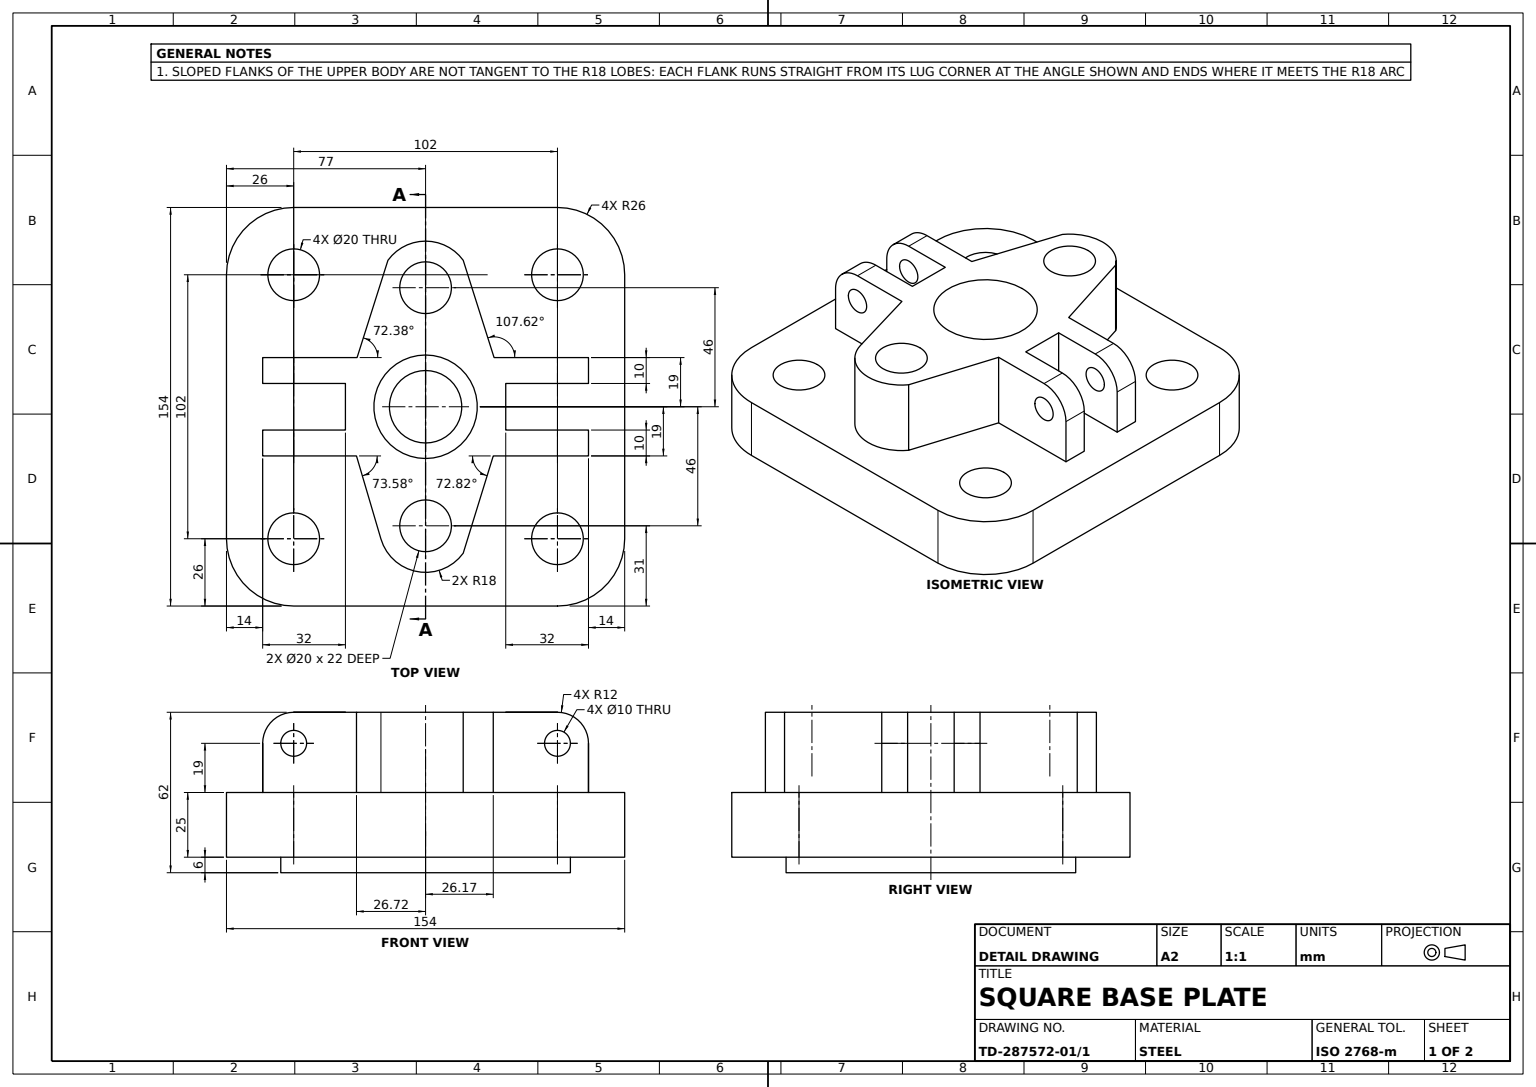
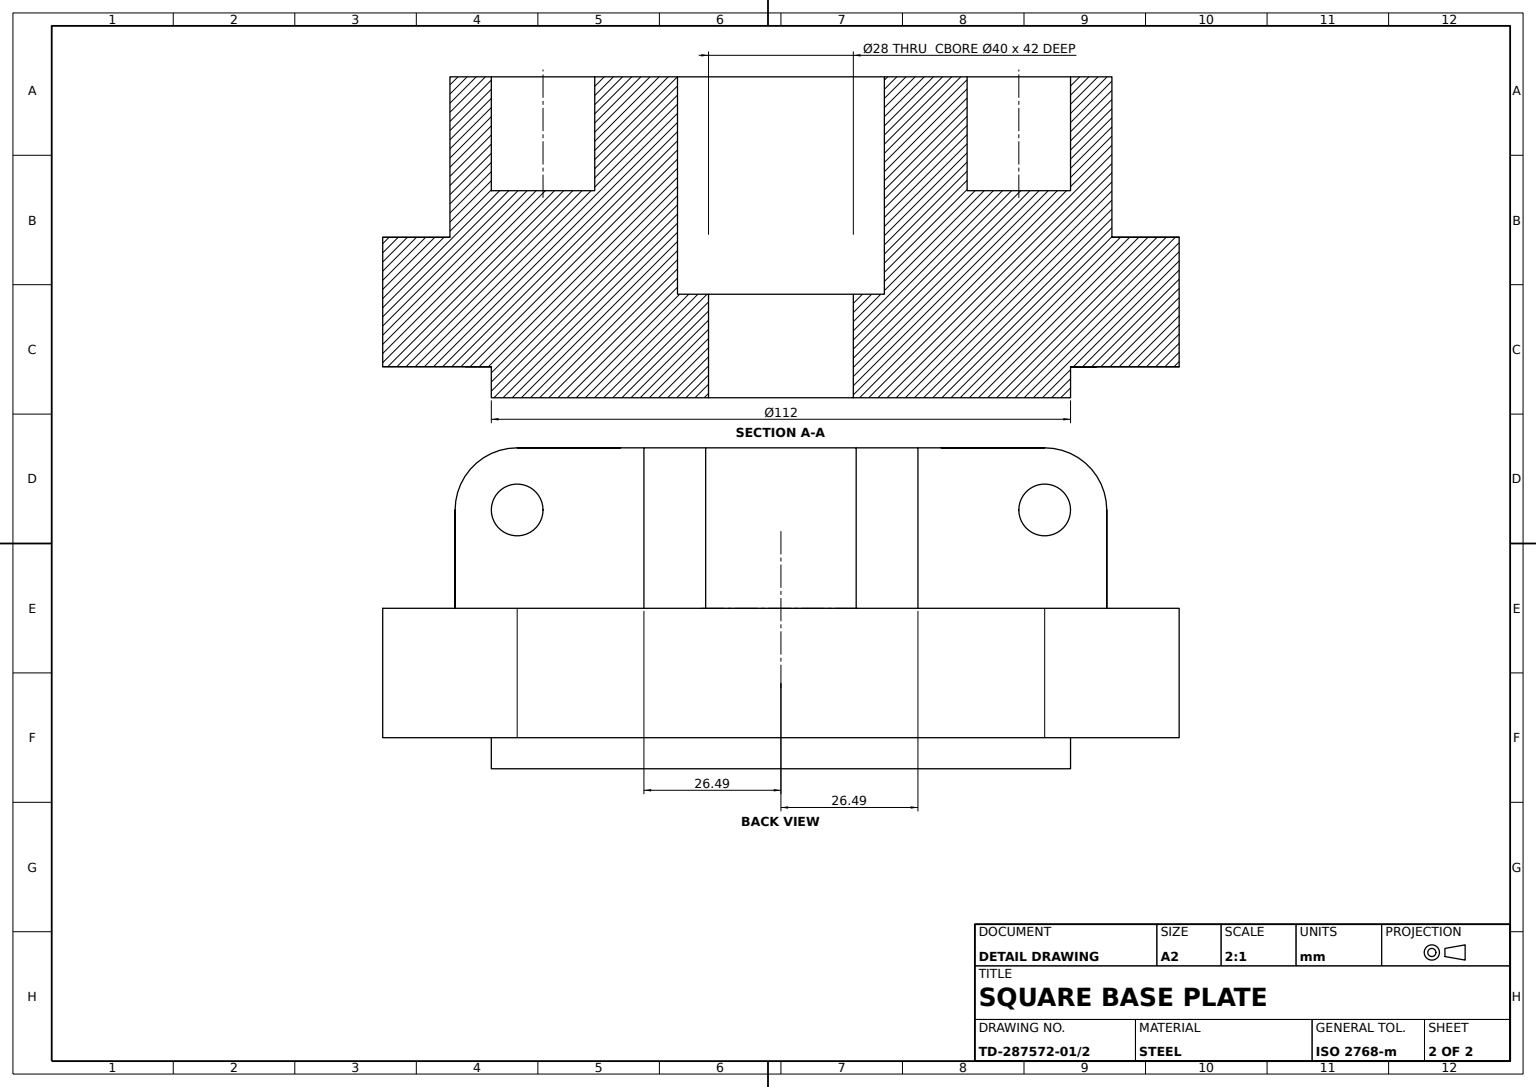
from build123d import *

# Parameters (mm, degrees)
BASE_PLATE_DEPTH              = 25
PLATE_MOUNTING_HOLES_SKETCH_R = 10
PLATE_MOUNTING_HOLES_DEPTH    = 112
CENTRAL_BOSS_DEPTH            = 31
LUG_START                     = -31
LUG_PAIR_A_DEPTH              = 31
LUG_PAIR_B_DEPTH              = 31
LUG_PIN_HOLES_SKETCH_R        = 5
LUG_PIN_HOLES_DEPTH           = 118
LUG_A_FILLET_1_R              = 12
LUG_A_FILLET_2_R              = 12
LUG_B_FILLET_1_R              = 12
LUG_B_FILLET_2_R              = 12
CENTRAL_BORE_SKETCH_R         = 14
CENTRAL_BORE_DEPTH            = 118
BORE_COUNTERBORE_SKETCH_R     = 20
BORE_COUNTERBORE_DEPTH        = 42
BOTTOM_SPIGOT_SKETCH_R        = 56
BOTTOM_SPIGOT_DEPTH           = 6
SPIGOT_BORE_SKETCH_R          = 14
SPIGOT_BORE_DEPTH             = 120
FLANGE_HOLE_1_SKETCH_R        = 10
FLANGE_HOLE_1_DEPTH           = 22
FLANGE_HOLE_2_SKETCH_R        = 10
FLANGE_HOLE_2_DEPTH           = 22


with BuildPart() as part:
    # Base Plate Sketch → Base Plate (new body)
    with BuildSketch(Plane(origin=(0, 0, 0), x_dir=(1, 0, 0), z_dir=(0, 1, 0))):
        with BuildLine():
            Line((77, 0), (77, 51))
            ThreePointArc((77, 51), (69.384776311, 69.384776311), (51, 77))
            Line((51, 77), (-51, 77))
            ThreePointArc((-51, 77), (-69.384776311, 69.384776311), (-77, 51))
            Line((-77, 51), (-77, -51))
            ThreePointArc((-77, -51), (-69.384776311, -69.384776311), (-51, -77))
            Line((-51, -77), (51, -77))
            ThreePointArc((51, -77), (69.384776311, -69.384776311), (77, -51))
            Line((77, -51), (77, 0))
        make_face()
    extrude(amount=BASE_PLATE_DEPTH)

    # Plate Mounting Holes Sketch → Plate Mounting Holes (cut)
    with BuildSketch(Plane(origin=(0, 25, 0), x_dir=(1, 0, 0), z_dir=(0, 1, 0))):
        with Locations(Location((-51, 51, 0), (0, 0, 270))):
            Circle(PLATE_MOUNTING_HOLES_SKETCH_R)
        with Locations(Location((51, 51, 0), (0, 0, 270))):
            Circle(PLATE_MOUNTING_HOLES_SKETCH_R)
        with Locations(Location((51, -51, 0), (0, 0, 270))):
            Circle(PLATE_MOUNTING_HOLES_SKETCH_R)
        with Locations(Location((-51, -51, 0), (0, 0, 270))):
            Circle(PLATE_MOUNTING_HOLES_SKETCH_R)
    extrude(amount=-PLATE_MOUNTING_HOLES_DEPTH, mode=Mode.SUBTRACT)

    # Central Boss Sketch → Central Boss (add)
    with BuildSketch(Plane(origin=(0, 25, 0), x_dir=(1, 0, 0), z_dir=(0, 1, 0))):
        with BuildLine():
            Line((14.551173168, 56.595440502), (29.545654505, 9.383725265))
            ThreePointArc((29.545654505, 9.383725265), (30.89470992, 2.552821763), (30.685167625, -4.406868258))
            Line((30.685167625, -4.406868258), (14.551173168, -56.595440502))
            ThreePointArc((14.551173168, -56.595440502), (-3.070625216, -63.736156878), (-17.266235066, -51.086956522))
            Line((-17.266235066, -51.086956522), (-29.736293724, -8.760869565))
            ThreePointArc((-29.736293724, -8.760869565), (-30.998289096, 0.325688707), (-29.545654505, 9.383725265))
            Line((-29.545654505, 9.383725265), (-14.551173168, 56.595440502))
            ThreePointArc((-14.551173168, 56.595440502), (0, 64), (14.551173168, 56.595440502))
        make_face()
    extrude(amount=CENTRAL_BOSS_DEPTH)

    # Lug Pair A Sketch → Lug Pair A (add)
    with BuildSketch(Plane(origin=(0, 56, 0), x_dir=(1, 0, 0), z_dir=(0, 1, 0)).offset(LUG_START)):
        with BuildLine():
            Line((31, 0), (31, 9))
            Line((31, 9), (63, 9))
            Line((63, 9), (63, 19))
            Line((63, 19), (31, 19))
            Line((31, 19), (26.491517384, 19))
            Line((26.491517384, 19), (29.545654505, 9.383725265))
            ThreePointArc((29.545654505, 9.383725265), (30.634256068, 4.747879018), (31, 0))
        make_face()
        with BuildLine():
            Line((31, -9), (31, 0))
            ThreePointArc((31, 0), (30.921191733, -2.209049981), (30.685167625, -4.406868258))
            ThreePointArc((30.685167625, -4.406868258), (29.6170045, -9.156038686), (27.818568264, -13.679446617))
            Line((27.818568264, -13.679446617), (26.173729651, -19))
            Line((26.173729651, -19), (31, -19))
            Line((31, -19), (63, -19))
            Line((63, -19), (63, -9))
            Line((63, -9), (31, -9))
        make_face()
        with BuildLine():
            ThreePointArc((24.494897428, 19), (27.444735347, 14.414801481), (29.545654505, 9.383725265))
            Line((29.545654505, 9.383725265), (26.491517384, 19))
            Line((26.491517384, 19), (24.494897428, 19))
        make_face()
        with BuildLine():
            Line((26.173729651, -19), (27.818568264, -13.679446617))
            ThreePointArc((27.818568264, -13.679446617), (26.29166684, -16.424014575), (24.494897428, -19))
            Line((24.494897428, -19), (26.173729651, -19))
        make_face()
        with BuildLine():
            ThreePointArc((27.818568264, -13.679446617), (29.6170045, -9.156038686), (30.685167625, -4.406868258))
            Line((30.685167625, -4.406868258), (27.818568264, -13.679446617))
        make_face()
    extrude(amount=LUG_PAIR_A_DEPTH)

    # Lug Pair B Sketch → Lug Pair B (add)
    with BuildSketch(Plane(origin=(0, 56, 0), x_dir=(1, 0, 0), z_dir=(0, 1, 0)).offset(LUG_START)):
        with BuildLine():
            ThreePointArc((-29.736293724, -8.760869565), (-30.682446981, -4.425770811), (-31, 0))
            Line((-31, 0), (-31, -9))
            Line((-31, -9), (-63, -9))
            Line((-63, -9), (-63, -19))
            Line((-63, -19), (-26.719653956, -19))
            Line((-26.719653956, -19), (-29.736293724, -8.760869565))
        make_face()
        with BuildLine():
            Line((-31, 9), (-31, 0))
            ThreePointArc((-31, 0), (-30.634256068, 4.747879018), (-29.545654505, 9.383725265))
            Line((-29.545654505, 9.383725265), (-26.491517384, 19))
            Line((-26.491517384, 19), (-63, 19))
            Line((-63, 19), (-63, 9))
            Line((-63, 9), (-31, 9))
        make_face()
        with BuildLine():
            ThreePointArc((-24.494897428, -19), (-27.594663822, -14.125669136), (-29.736293724, -8.760869565))
            Line((-29.736293724, -8.760869565), (-26.719653956, -19))
            Line((-26.719653956, -19), (-24.494897428, -19))
        make_face()
        with BuildLine():
            Line((-26.491517384, 19), (-29.545654505, 9.383725265))
            ThreePointArc((-29.545654505, 9.383725265), (-27.444735347, 14.414801481), (-24.494897428, 19))
            Line((-24.494897428, 19), (-26.491517384, 19))
        make_face()
    extrude(amount=LUG_PAIR_B_DEPTH)

    # Lug Pin Holes Sketch → Lug Pin Holes (cut)
    with BuildSketch(Plane.XY.offset(19)):
        with Locations((51, 44)):
            Circle(LUG_PIN_HOLES_SKETCH_R)
        with Locations((-51, 44)):
            Circle(LUG_PIN_HOLES_SKETCH_R)
    extrude(amount=-LUG_PIN_HOLES_DEPTH, mode=Mode.SUBTRACT)

    # Lug A Fillet 1
    lug_a_fillet_1_edges = [part.edges().sort_by_distance(p)[0] for p in [
        (63, 56, 14),
    ]]
    fillet(lug_a_fillet_1_edges, radius=LUG_A_FILLET_1_R)

    # Lug A Fillet 2
    lug_a_fillet_2_edges = [part.edges().sort_by_distance(p)[0] for p in [
        (63, 56, -14),
    ]]
    fillet(lug_a_fillet_2_edges, radius=LUG_A_FILLET_2_R)

    # Lug B Fillet 1
    lug_b_fillet_1_edges = [part.edges().sort_by_distance(p)[0] for p in [
        (-63, 56, -14),
    ]]
    fillet(lug_b_fillet_1_edges, radius=LUG_B_FILLET_1_R)

    # Lug B Fillet 2
    lug_b_fillet_2_edges = [part.edges().sort_by_distance(p)[0] for p in [
        (-63, 56, 14),
    ]]
    fillet(lug_b_fillet_2_edges, radius=LUG_B_FILLET_2_R)

    # Central Bore Sketch → Central Bore (cut)
    with BuildSketch(Plane(origin=(0, 56, 0), x_dir=(1, 0, 0), z_dir=(0, 1, 0))):
        with Locations(Location((0, 0, 0), (0, 0, 270))):
            Circle(CENTRAL_BORE_SKETCH_R)
    extrude(amount=-CENTRAL_BORE_DEPTH, mode=Mode.SUBTRACT)

    # Bore Counterbore Sketch → Bore Counterbore (cut)
    with BuildSketch(Plane(origin=(0, 56, 0), x_dir=(1, 0, 0), z_dir=(0, 1, 0))):
        with Locations(Location((0, 0, 0), (0, 0, 270))):
            Circle(BORE_COUNTERBORE_SKETCH_R)
    extrude(amount=-BORE_COUNTERBORE_DEPTH, mode=Mode.SUBTRACT)

    # Bottom Spigot Sketch → Bottom Spigot (add)
    with BuildSketch(Plane.XZ):
        with Locations(Location((0, 0, 0), (0, 0, 270))):
            Circle(BOTTOM_SPIGOT_SKETCH_R)
    extrude(amount=BOTTOM_SPIGOT_DEPTH)

    # Spigot Bore Sketch → Spigot Bore (cut)
    with BuildSketch(Plane(origin=(0, 0, 0), x_dir=(1, 0, 0), z_dir=(0, 1, 0))):
        with Locations(Location((0, 0, 0), (0, 0, 270))):
            Circle(SPIGOT_BORE_SKETCH_R)
    extrude(amount=-SPIGOT_BORE_DEPTH, mode=Mode.SUBTRACT)

    # Flange Hole 1 Sketch → Flange Hole 1 (cut)
    with BuildSketch(Plane(origin=(0, 56, 0), x_dir=(1, 0, 0), z_dir=(0, 1, 0))):
        with Locations(Location((0, 46, 0), (0, 0, 270))):
            Circle(FLANGE_HOLE_1_SKETCH_R)
    extrude(amount=-FLANGE_HOLE_1_DEPTH, mode=Mode.SUBTRACT)

    # Flange Hole 2 Sketch → Flange Hole 2 (cut)
    with BuildSketch(Plane(origin=(0, 56, 0), x_dir=(1, 0, 0), z_dir=(0, 1, 0))):
        with Locations(Location((0, -46, 0), (0, 0, 270))):
            Circle(FLANGE_HOLE_2_SKETCH_R)
    extrude(amount=-FLANGE_HOLE_2_DEPTH, mode=Mode.SUBTRACT)


solid = part.part
